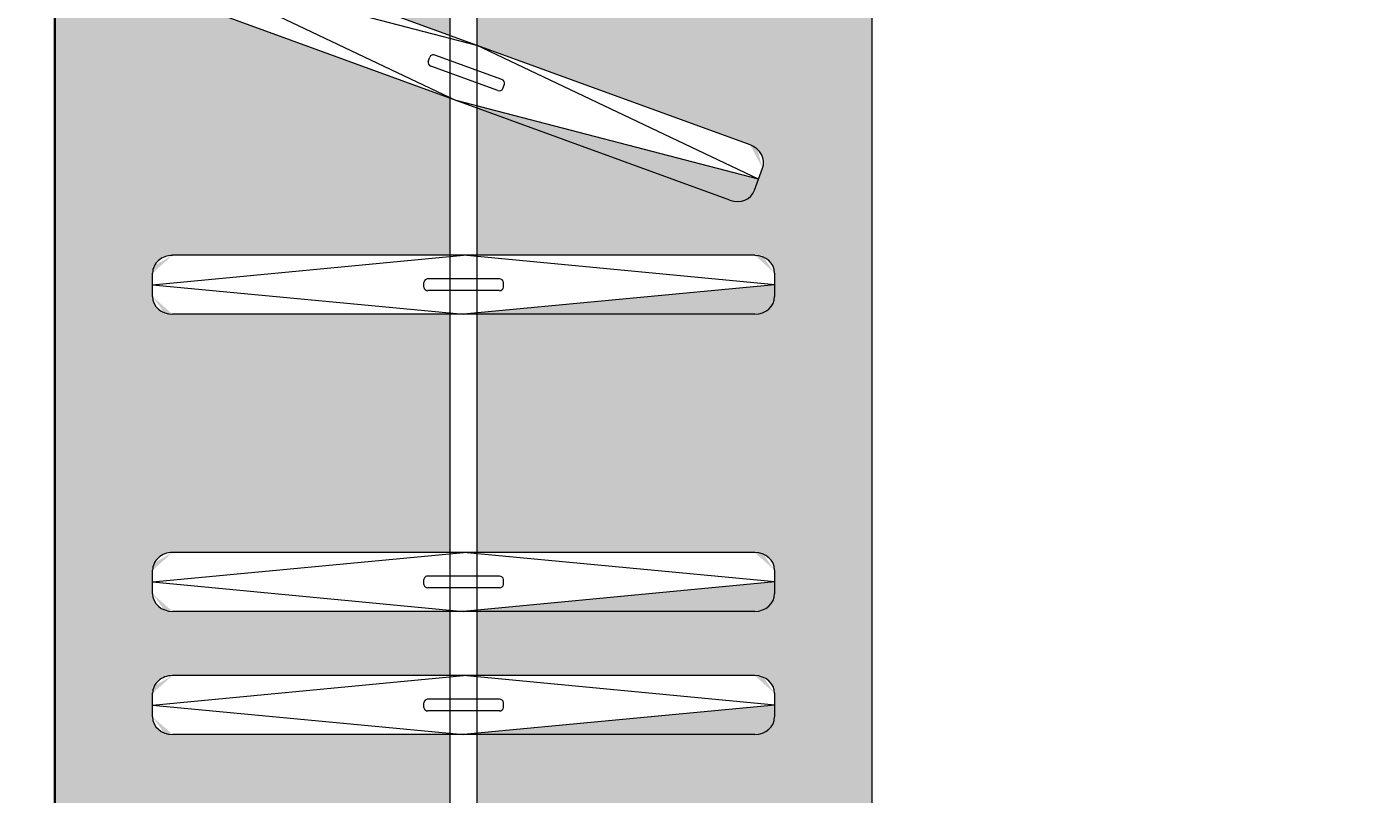
# Model space of a CAD drawing. Units: millimetres. Extents: x 27017497 to 27018854, y 7058029 to 7059154.
# Tile 66 of 91: x 27018319 to 27018355, y 7058154 to 7058174. Entities that reach past the tile are written whole.
import ezdxf

# ---------------------------------------------------------------- set-up
doc = ezdxf.new("R2010")
doc.units = ezdxf.units.MM
for name, color, linetype, lineweight in [('A-ANNO-DIMS', 2, 'Continuous', 18), ('A-FLOR-CASE', 8, 'Continuous', 20), ('A-FLOR-CASE-PATT', 44, 'Continuous', 13), ('A-WALL', 7, 'Continuous', 35)]:
    doc.layers.add(name, color=color, linetype=linetype, lineweight=lineweight)
doc.styles.get("Standard").update_dxf_attribs({"font": 'arial.ttf'})
doc.dimstyles.get("Standard").update_dxf_attribs({"dimtxt": 0.18, "dimasz": 0.18, "dimexe": 0.18, "dimexo": 0.0625, "dimgap": 0.09, "dimtad": 0, "dimtih": 1, "dimtoh": 1, "dimdec": 4, "dimzin": 0, "dimdsep": 46, "dimtxsty": 'Standard', "dimcen": 0.09, "dimadec": 0, "dimazin": 0, "dimtfac": 1, "dimtdec": 4, "dimtofl": 0, "dimtmove": 0, "dimatfit": 3, "dimfxl": 1, "dimtolj": 1, "dimtzin": 0, "dimarcsym": 0})

# ---------------------------------------------------------------- blocks, each defined once
blk = doc.blocks.new('WARDROBE-HANGING')
for p, q in [((0, 21.737), (65.212, 21.737)), ((39.589, 19.153), (38.806, 10.877)), ((39.902, 19.153), (39.276, 19.153)), ((39.589, 19.153), (40.372, 10.877)), ((47.493, 19.153), (46.71, 10.877)), ((47.806, 19.153), (47.18, 19.153)), ((47.493, 19.153), (48.276, 10.877)), ((50.766, 19.153), (49.984, 10.877)), ((51.079, 19.153), (50.453, 19.153)), ((50.766, 19.153), (51.549, 10.877)), ((36.783, 18.726), (33.217, 11.217)), ((36.783, 18.726), (34.688, 10.682)), ((37.077, 18.619), (36.488, 18.833)), ((38.806, 18.624), (38.806, 3.13)), ((40.372, 18.624), (40.372, 3.13)), ((46.71, 18.624), (46.71, 3.13)), ((48.276, 18.624), (48.276, 3.13)), ((49.984, 18.624), (49.984, 3.13)), ((51.549, 18.624), (51.549, 3.13)), ((35.867, 18.497), (30.567, 3.937)), ((37.337, 17.962), (32.038, 3.402)), ((34.13, 11.896), (33.48, 10.11)), ((34.372, 11.921), (34.255, 11.964)), ((39.432, 11.828), (39.432, 9.927)), ((39.652, 11.934), (39.526, 11.934)), ((39.745, 11.828), (39.745, 9.927)), ((47.336, 11.828), (47.336, 9.927)), ((47.556, 11.934), (47.43, 11.934)), ((47.649, 11.828), (47.649, 9.927)), ((50.61, 11.828), (50.61, 9.927)), ((50.829, 11.934), (50.704, 11.934)), ((50.923, 11.828), (50.923, 9.927)), ((34.425, 11.789), (33.774, 10.002)), ((0, 11.231), (65.212, 11.231)), ((31.122, 3.173), (33.217, 11.217)), ((39.589, 2.602), (38.806, 10.877)), ((39.589, 2.602), (40.372, 10.877)), ((47.493, 2.602), (46.71, 10.877)), ((47.493, 2.602), (48.276, 10.877)), ((50.766, 2.602), (49.984, 10.877)), ((50.766, 2.602), (51.549, 10.877)), ((0, 10.506), (65.212, 10.506)), ((31.122, 3.173), (34.688, 10.682)), ((33.65, 9.935), (33.532, 9.978)), ((39.652, 9.821), (39.526, 9.821)), ((47.556, 9.821), (47.43, 9.821)), ((50.829, 9.821), (50.704, 9.821)), ((39.902, 2.602), (39.276, 2.602)), ((47.806, 2.602), (47.18, 2.602)), ((51.079, 2.602), (50.453, 2.602)), ((0, 0), (65.212, 0))]:
    blk.add_line(p, q)
for centre, major_axis, start_param, end_param in [((39.276, 18.624), (0, 0.528), 0, 1.570796), ((39.902, 18.624), (0, 0.528), 4.712389, 6.283185), ((47.18, 18.624), (0, 0.528), 0, 1.570796), ((47.806, 18.624), (0, 0.528), 4.712389, 6.283185), ((50.453, 18.624), (0, 0.528), 0, 1.570796), ((51.079, 18.624), (0, 0.528), 4.712389, 6.283185), ((36.308, 18.336), (0.181, 0.496), 0, 1.570796), ((36.896, 18.122), (0.181, 0.496), -1.570796, 0), ((34.219, 11.864), (0.0361, 0.0993), 0, 1.570796), ((34.336, 11.821), (0.0361, 0.0993), 4.712389, 6.283185), ((39.526, 11.828), (0, 0.106), 0, 1.570796), ((39.652, 11.828), (0, 0.106), -1.570796, 0), ((47.43, 11.828), (0, 0.106), 0, 1.570796), ((47.556, 11.828), (0, 0.106), -1.570796, 0), ((50.704, 11.828), (0, 0.106), 0, 1.570796), ((50.829, 11.828), (0, 0.106), -1.570796, 0), ((33.568, 10.077), (0.0361, 0.0993), 1.570796, 3.141593), ((33.686, 10.035), (0.0361, 0.0993), 3.141593, 4.712389), ((39.526, 9.927), (0, 0.106), 1.570796, 3.141593), ((39.652, 9.927), (0, 0.106), 3.141593, 4.712389), ((47.43, 9.927), (0, 0.106), 1.570796, 3.141593), ((47.556, 9.927), (0, 0.106), 3.141593, 4.712389), ((50.704, 9.927), (0, 0.106), 1.570796, 3.141593), ((50.829, 9.927), (0, 0.106), 3.141593, 4.712389), ((39.276, 3.13), (0, 0.528), 1.570796, 3.141593), ((39.902, 3.13), (0, 0.528), 3.141593, 4.712389), ((47.18, 3.13), (0, 0.528), 1.570796, 3.141593), ((47.806, 3.13), (0, 0.528), 3.141593, 4.712389), ((50.453, 3.13), (0, 0.528), 1.570796, 3.141593), ((51.079, 3.13), (0, 0.528), 3.141593, 4.712389)]:
    blk.add_ellipse(centre, major_axis=major_axis, ratio=0.888892, start_param=start_param, end_param=end_param)
blk = doc.blocks.new('*D33')
at = {"layer": 'A-ANNO-DIMS', "color": 0, "lineweight": -2, "transparency": 16777216}
for p, q in [((27018319.543, 7058207.1), (27018309.644, 7058207.1)), ((27018309.824, 7058206.92), (27018309.824, 7058174.677)), ((27018309.824, 7058142.068), (27018309.824, 7058174.311)), ((27018319.543, 7058141.888), (27018309.644, 7058141.888))]:
    blk.add_line(p, q, dxfattribs=at)
at = {"layer": 'A-ANNO-DIMS', "color": 0, "transparency": 16777216}
for points in [[(27018309.794, 7058206.92), (27018309.854, 7058206.92), (27018309.824, 7058207.1)], [(27018309.794, 7058142.068), (27018309.854, 7058142.068), (27018309.824, 7058141.888)]]:
    blk.add_solid(points, dxfattribs=at)
at = {"layer": 'Defpoints', "color": 0, "transparency": 16777216}
for p in [(27018319.606, 7058207.1), (27018309.824, 7058141.888), (27018319.606, 7058141.888)]:
    blk.add_point(p, dxfattribs=at)
at = {"layer": 'A-ANNO-DIMS', "color": 0, "transparency": 16777216, "insert": (27018309.824, 7058174.494), "char_height": 0.18, "attachment_point": 5}
blk.add_mtext('\\A1;WARDROBE 65 TYP.', dxfattribs=at)
blk = doc.blocks.new('*D47')
at = {"layer": 'A-ANNO-DIMS', "color": 0, "lineweight": -2, "transparency": 16777216}
for p, q in [((27017561.166, 7058294.35), (27017561.166, 7058028.6)), ((27018790.606, 7058294.35), (27018790.606, 7058028.6)), ((27017561.346, 7058028.78), (27018175.431, 7058028.78)), ((27018790.426, 7058028.78), (27018176.341, 7058028.78))]:
    blk.add_line(p, q, dxfattribs=at)
at = {"layer": 'A-ANNO-DIMS', "color": 0, "transparency": 16777216}
for points in [[(27017561.346, 7058028.81), (27017561.346, 7058028.75), (27017561.166, 7058028.78)], [(27018790.426, 7058028.81), (27018790.426, 7058028.75), (27018790.606, 7058028.78)]]:
    blk.add_solid(points, dxfattribs=at)
at = {"layer": 'Defpoints', "color": 0, "transparency": 16777216}
for p in [(27017561.166, 7058294.412), (27018790.606, 7058294.412), (27018790.606, 7058028.78)]:
    blk.add_point(p, dxfattribs=at)
at = {"layer": 'A-ANNO-DIMS', "color": 0, "transparency": 16777216, "insert": (27018175.886, 7058028.78), "char_height": 0.18, "attachment_point": 5}
blk.add_mtext('\\A1;1229.4', dxfattribs=at)
blk = doc.blocks.new('*D48')
at = {"layer": 'A-ANNO-DIMS', "color": 0, "lineweight": -2, "transparency": 16777216}
for p, q in [((27018463.498, 7058622.912), (27017497.536, 7058622.912)), ((27017497.716, 7058622.732), (27017497.716, 7058357.753)), ((27017497.716, 7058092.41), (27017497.716, 7058357.389)), ((27018555.129, 7058092.23), (27017497.536, 7058092.23))]:
    blk.add_line(p, q, dxfattribs=at)
at = {"layer": 'A-ANNO-DIMS', "color": 0, "transparency": 16777216}
for points in [[(27017497.686, 7058622.732), (27017497.746, 7058622.732), (27017497.716, 7058622.912)], [(27017497.686, 7058092.41), (27017497.746, 7058092.41), (27017497.716, 7058092.23)]]:
    blk.add_solid(points, dxfattribs=at)
at = {"layer": 'Defpoints', "color": 0, "transparency": 16777216}
for p in [(27018463.561, 7058622.912), (27017497.716, 7058092.23), (27018555.192, 7058092.23)]:
    blk.add_point(p, dxfattribs=at)
at = {"layer": 'A-ANNO-DIMS', "color": 0, "transparency": 16777216, "insert": (27017497.716, 7058357.571), "char_height": 0.18, "attachment_point": 5}
blk.add_mtext('\\A1;530.7', dxfattribs=at)

msp = doc.modelspace()

# ---------------------------------------------------------------- hatches: boundary and pattern name
at = {"layer": 'A-FLOR-CASE-PATT'}
h = msp.add_hatch(color=256, dxfattribs=at)
h.dxf.hatch_style = 1
edge = h.paths.add_edge_path()
edge.add_line((27018341.343, 7058207.055), (27018330.837, 7058207.055))
edge.add_line((27018330.837, 7058207.055), (27018330.837, 7058203.02))
edge.add_line((27018330.837, 7058203.02), (27018338.424, 7058203.02))
edge.add_ellipse((27018338.23, 7058202.551), major_axis=(0.528, 0), ratio=0.888892, start_angle=0, end_angle=90, ccw=False)
edge.add_line((27018338.758, 7058202.551), (27018338.758, 7058202.238))
edge.add_line((27018338.758, 7058202.238), (27018330.837, 7058201.488))
edge.add_line((27018330.837, 7058201.488), (27018330.837, 7058199.747))
edge.add_line((27018330.837, 7058199.747), (27018338.424, 7058199.747))
edge.add_ellipse((27018338.23, 7058199.277), major_axis=(0.528, 0), ratio=0.888892, start_angle=0, end_angle=90, ccw=False)
edge.add_line((27018338.758, 7058199.277), (27018338.758, 7058198.964))
edge.add_line((27018338.758, 7058198.964), (27018330.837, 7058198.215))
edge.add_line((27018330.837, 7058198.215), (27018330.837, 7058193.415))
edge.add_line((27018330.837, 7058193.415), (27018338.284, 7058190.704))
edge.add_ellipse((27018337.942, 7058190.329), major_axis=(0.496, -0.181), ratio=0.888892, start_angle=0, end_angle=90, ccw=False)
edge.add_line((27018338.439, 7058190.148), (27018338.331, 7058189.854))
edge.add_line((27018338.331, 7058189.854), (27018330.837, 7058191.806))
edge.add_line((27018330.837, 7058191.806), (27018330.837, 7058188.22))
edge.add_line((27018330.837, 7058188.22), (27018338.424, 7058188.22))
edge.add_ellipse((27018338.23, 7058187.75), major_axis=(0.528, 0), ratio=0.888892, start_angle=0, end_angle=90, ccw=False)
edge.add_line((27018338.758, 7058187.75), (27018338.758, 7058187.437))
edge.add_line((27018338.758, 7058187.437), (27018330.837, 7058186.688))
edge.add_line((27018330.837, 7058186.688), (27018330.837, 7058181.982))
edge.add_line((27018330.837, 7058181.982), (27018338.424, 7058181.982))
edge.add_ellipse((27018338.23, 7058181.513), major_axis=(0.528, 0), ratio=0.888892, start_angle=0, end_angle=90, ccw=False)
edge.add_line((27018338.758, 7058181.513), (27018338.758, 7058181.199))
edge.add_line((27018338.758, 7058181.199), (27018330.837, 7058180.45))
edge.add_line((27018330.837, 7058180.45), (27018330.837, 7058178.709))
edge.add_line((27018330.837, 7058178.709), (27018338.424, 7058178.709))
edge.add_ellipse((27018338.23, 7058178.239), major_axis=(0.528, 0), ratio=0.888892, start_angle=0, end_angle=90, ccw=False)
edge.add_line((27018338.758, 7058178.239), (27018338.758, 7058177.926))
edge.add_line((27018338.758, 7058177.926), (27018330.837, 7058177.177))
edge.add_line((27018330.837, 7058177.177), (27018330.837, 7058173.878))
edge.add_line((27018330.837, 7058173.878), (27018338.284, 7058171.167))
edge.add_ellipse((27018337.942, 7058170.792), major_axis=(0.496, -0.181), ratio=0.888892, start_angle=0, end_angle=90, ccw=False)
edge.add_line((27018338.439, 7058170.611), (27018338.331, 7058170.317))
edge.add_line((27018338.331, 7058170.317), (27018330.837, 7058172.269))
edge.add_line((27018330.837, 7058172.269), (27018330.837, 7058168.293))
edge.add_line((27018330.837, 7058168.293), (27018338.424, 7058168.293))
edge.add_ellipse((27018338.23, 7058167.824), major_axis=(0.528, 0), ratio=0.888892, start_angle=0, end_angle=90, ccw=False)
edge.add_line((27018338.758, 7058167.824), (27018338.758, 7058167.511))
edge.add_line((27018338.758, 7058167.511), (27018330.837, 7058166.762))
edge.add_line((27018330.837, 7058166.762), (27018330.837, 7058160.389))
edge.add_line((27018330.837, 7058160.389), (27018338.424, 7058160.389))
edge.add_ellipse((27018338.23, 7058159.92), major_axis=(0.528, 0), ratio=0.888892, start_angle=0, end_angle=90, ccw=False)
edge.add_line((27018338.758, 7058159.92), (27018338.758, 7058159.607))
edge.add_line((27018338.758, 7058159.607), (27018330.837, 7058158.858))
edge.add_line((27018330.837, 7058158.858), (27018330.837, 7058157.116))
edge.add_line((27018330.837, 7058157.116), (27018338.424, 7058157.116))
edge.add_ellipse((27018338.23, 7058156.647), major_axis=(0.528, 0), ratio=0.888892, start_angle=0, end_angle=90, ccw=False)
edge.add_line((27018338.758, 7058156.647), (27018338.758, 7058156.334))
edge.add_line((27018338.758, 7058156.334), (27018330.837, 7058155.585))
edge.add_line((27018330.837, 7058155.585), (27018330.837, 7058150.784))
edge.add_line((27018330.837, 7058150.784), (27018338.284, 7058148.073))
edge.add_ellipse((27018337.942, 7058147.698), major_axis=(0.496, -0.181), ratio=0.888892, start_angle=0, end_angle=90, ccw=False)
edge.add_line((27018338.439, 7058147.517), (27018338.331, 7058147.223))
edge.add_line((27018338.331, 7058147.223), (27018330.837, 7058149.175))
edge.add_line((27018330.837, 7058149.175), (27018330.837, 7058145.589))
edge.add_line((27018330.837, 7058145.589), (27018338.424, 7058145.589))
edge.add_ellipse((27018338.23, 7058145.119), major_axis=(0.528, 0), ratio=0.888892, start_angle=0, end_angle=90, ccw=False)
edge.add_line((27018338.758, 7058145.119), (27018338.758, 7058144.806))
edge.add_line((27018338.758, 7058144.806), (27018330.837, 7058144.057))
edge.add_line((27018330.837, 7058144.057), (27018330.837, 7058141.912))
edge.add_line((27018330.837, 7058141.912), (27018341.343, 7058141.912))
edge.add_line((27018341.343, 7058141.912), (27018341.343, 7058207.055))
edge = h.paths.add_edge_path()
edge.add_line((27018330.112, 7058207.055), (27018319.606, 7058207.055))
edge.add_line((27018319.606, 7058207.055), (27018319.606, 7058141.912))
edge.add_line((27018319.606, 7058141.912), (27018330.112, 7058141.912))
edge.add_line((27018330.112, 7058141.912), (27018330.112, 7058144.024))
edge.add_line((27018330.112, 7058144.024), (27018322.543, 7058144.024))
edge.add_ellipse((27018322.736, 7058144.493), major_axis=(0.528, 0), ratio=0.888892, start_angle=180, end_angle=270, ccw=False)
edge.add_line((27018322.208, 7058144.493), (27018322.208, 7058145.291))
edge.add_ellipse((27018322.736, 7058145.119), major_axis=(0.528, 0), ratio=0.888892, start_angle=90, end_angle=180, ccw=False)
edge.add_line((27018322.736, 7058145.589), (27018330.112, 7058145.589))
edge.add_line((27018330.112, 7058145.589), (27018330.112, 7058149.382))
edge.add_line((27018330.112, 7058149.382), (27018322.826, 7058152.034))
edge.add_ellipse((27018323.168, 7058152.409), major_axis=(0.496, -0.181), ratio=0.888892, start_angle=180, end_angle=270, ccw=False)
edge.add_line((27018322.672, 7058152.59), (27018322.945, 7058153.34))
edge.add_ellipse((27018323.382, 7058152.997), major_axis=(0.496, -0.181), ratio=0.888892, start_angle=90, end_angle=180, ccw=False)
edge.add_line((27018323.543, 7058153.439), (27018330.112, 7058151.048))
edge.add_line((27018330.112, 7058151.048), (27018330.112, 7058155.551))
edge.add_line((27018330.112, 7058155.551), (27018322.543, 7058155.551))
edge.add_ellipse((27018322.736, 7058156.021), major_axis=(0.528, 0), ratio=0.888892, start_angle=180, end_angle=270, ccw=False)
edge.add_line((27018322.208, 7058156.021), (27018322.208, 7058156.819))
edge.add_ellipse((27018322.736, 7058156.647), major_axis=(0.528, 0), ratio=0.888892, start_angle=90, end_angle=180, ccw=False)
edge.add_line((27018322.736, 7058157.116), (27018330.112, 7058157.116))
edge.add_line((27018330.112, 7058157.116), (27018330.112, 7058158.824))
edge.add_line((27018330.112, 7058158.824), (27018322.543, 7058158.824))
edge.add_ellipse((27018322.736, 7058159.294), major_axis=(0.528, 0), ratio=0.888892, start_angle=180, end_angle=270, ccw=False)
edge.add_line((27018322.208, 7058159.294), (27018322.208, 7058160.092))
edge.add_ellipse((27018322.736, 7058159.92), major_axis=(0.528, 0), ratio=0.888892, start_angle=90, end_angle=180, ccw=False)
edge.add_line((27018322.736, 7058160.389), (27018330.112, 7058160.389))
edge.add_line((27018330.112, 7058160.389), (27018330.112, 7058166.728))
edge.add_line((27018330.112, 7058166.728), (27018322.543, 7058166.728))
edge.add_ellipse((27018322.736, 7058167.198), major_axis=(0.528, 0), ratio=0.888892, start_angle=180, end_angle=270, ccw=False)
edge.add_line((27018322.208, 7058167.198), (27018322.208, 7058167.996))
edge.add_ellipse((27018322.736, 7058167.824), major_axis=(0.528, 0), ratio=0.888892, start_angle=90, end_angle=180, ccw=False)
edge.add_line((27018322.736, 7058168.293), (27018330.112, 7058168.293))
edge.add_line((27018330.112, 7058168.293), (27018330.112, 7058172.476))
edge.add_line((27018330.112, 7058172.476), (27018322.826, 7058175.128))
edge.add_ellipse((27018323.168, 7058175.503), major_axis=(0.496, -0.181), ratio=0.888892, start_angle=180, end_angle=270, ccw=False)
edge.add_line((27018322.672, 7058175.684), (27018322.945, 7058176.433))
edge.add_ellipse((27018323.382, 7058176.091), major_axis=(0.496, -0.181), ratio=0.888892, start_angle=90, end_angle=180, ccw=False)
edge.add_line((27018323.543, 7058176.533), (27018330.112, 7058174.142))
edge.add_line((27018330.112, 7058174.142), (27018330.112, 7058177.144))
edge.add_line((27018330.112, 7058177.144), (27018322.543, 7058177.144))
edge.add_ellipse((27018322.736, 7058177.613), major_axis=(0.528, 0), ratio=0.888892, start_angle=180, end_angle=270, ccw=False)
edge.add_line((27018322.208, 7058177.613), (27018322.208, 7058178.411))
edge.add_ellipse((27018322.736, 7058178.239), major_axis=(0.528, 0), ratio=0.888892, start_angle=90, end_angle=180, ccw=False)
edge.add_line((27018322.736, 7058178.709), (27018330.112, 7058178.709))
edge.add_line((27018330.112, 7058178.709), (27018330.112, 7058180.417))
edge.add_line((27018330.112, 7058180.417), (27018322.543, 7058180.417))
edge.add_ellipse((27018322.736, 7058180.886), major_axis=(0.528, 0), ratio=0.888892, start_angle=180, end_angle=270, ccw=False)
edge.add_line((27018322.208, 7058180.886), (27018322.208, 7058181.684))
edge.add_ellipse((27018322.736, 7058181.513), major_axis=(0.528, 0), ratio=0.888892, start_angle=90, end_angle=180, ccw=False)
edge.add_line((27018322.736, 7058181.982), (27018330.112, 7058181.982))
edge.add_line((27018330.112, 7058181.982), (27018330.112, 7058186.655))
edge.add_line((27018330.112, 7058186.655), (27018322.543, 7058186.655))
edge.add_ellipse((27018322.736, 7058187.124), major_axis=(0.528, 0), ratio=0.888892, start_angle=180, end_angle=270, ccw=False)
edge.add_line((27018322.208, 7058187.124), (27018322.208, 7058187.922))
edge.add_ellipse((27018322.736, 7058187.75), major_axis=(0.528, 0), ratio=0.888892, start_angle=90, end_angle=180, ccw=False)
edge.add_line((27018322.736, 7058188.22), (27018330.112, 7058188.22))
edge.add_line((27018330.112, 7058188.22), (27018330.112, 7058192.013))
edge.add_line((27018330.112, 7058192.013), (27018322.826, 7058194.665))
edge.add_ellipse((27018323.168, 7058195.04), major_axis=(0.496, -0.181), ratio=0.888892, start_angle=180, end_angle=270, ccw=False)
edge.add_line((27018322.672, 7058195.22), (27018322.945, 7058195.97))
edge.add_ellipse((27018323.382, 7058195.628), major_axis=(0.496, -0.181), ratio=0.888892, start_angle=90, end_angle=180, ccw=False)
edge.add_line((27018323.543, 7058196.069), (27018330.112, 7058193.678))
edge.add_line((27018330.112, 7058193.678), (27018330.112, 7058198.182))
edge.add_line((27018330.112, 7058198.182), (27018322.543, 7058198.182))
edge.add_ellipse((27018322.736, 7058198.651), major_axis=(0.528, 0), ratio=0.888892, start_angle=180, end_angle=270, ccw=False)
edge.add_line((27018322.208, 7058198.651), (27018322.208, 7058199.449))
edge.add_ellipse((27018322.736, 7058199.277), major_axis=(0.528, 0), ratio=0.888892, start_angle=90, end_angle=180, ccw=False)
edge.add_line((27018322.736, 7058199.747), (27018330.112, 7058199.747))
edge.add_line((27018330.112, 7058199.747), (27018330.112, 7058201.455))
edge.add_line((27018330.112, 7058201.455), (27018322.543, 7058201.455))
edge.add_ellipse((27018322.736, 7058201.924), major_axis=(0.528, 0), ratio=0.888892, start_angle=180, end_angle=270, ccw=False)
edge.add_line((27018322.208, 7058201.924), (27018322.208, 7058202.722))
edge.add_ellipse((27018322.736, 7058202.551), major_axis=(0.528, 0), ratio=0.888892, start_angle=90, end_angle=180, ccw=False)
edge.add_line((27018322.736, 7058203.02), (27018330.112, 7058203.02))
edge.add_line((27018330.112, 7058203.02), (27018330.112, 7058207.055))
h.paths.add_polyline_path([(27018341.31, 7058294.412), (27018319.606, 7058294.412), (27018319.606, 7058207.1), (27018341.31, 7058207.1)])
h.paths.add_polyline_path([(27018354.358, 7058255.592), (27018354.358, 7058256.057, -0.414214), (27018354.869, 7058256.569), (27018346.477, 7058256.569, -0.414214), (27018345.197, 7058257.848), (27018345.197, 7058259.128, -0.414214), (27018346.477, 7058260.407), (27018343.868, 7058260.407, 0.290979), (27018341.551, 7058258.934), (27018341.551, 7058242.534, 0.290979), (27018343.868, 7058241.06), (27018346.477, 7058241.06, -0.414214), (27018345.197, 7058242.34), (27018345.197, 7058243.619, -0.414214), (27018346.477, 7058244.899), (27018353.078, 7058244.899, 0.414214), (27018354.358, 7058246.178)])
h.paths.add_polyline_path([(27018356.917, 7058260.407), (27018346.477, 7058260.407, 0.414214), (27018345.197, 7058259.128), (27018345.197, 7058257.848, 0.414214), (27018346.477, 7058256.569), (27018355.637, 7058256.569), (27018355.637, 7058244.899), (27018346.477, 7058244.899, 0.414214), (27018345.197, 7058243.619), (27018345.197, 7058242.34, 0.414214), (27018346.477, 7058241.06), (27018356.917, 7058241.06, 0.414214), (27018359.476, 7058243.619), (27018359.476, 7058257.848, 0.414214)])
h.paths.add_polyline_path([(27018355.637, 7058252.362), (27018355.637, 7058256.057, 0.490314), (27018354.997, 7058256.553, 0.490314), (27018354.358, 7058256.057), (27018354.358, 7058255.592), (27018354.358, 7058245.411, 0.490314), (27018354.997, 7058244.915, 0.490314), (27018355.637, 7058245.411)], flags=17)

# ---------------------------------------------------------------- linework, layer by layer
at = {"layer": 'A-WALL'}
msp.add_line((27018319.606, 7058386.803), (27018319.606, 7058141.912), dxfattribs=at)

# ---------------------------------------------------------------- block references
at = {"layer": 'A-FLOR-CASE', "rotation": 270}
msp.add_blockref('WARDROBE-HANGING', (27018319.606, 7058207.1), dxfattribs=at)

# ---------------------------------------------------------------- dimensions: what is measured, and where the dimension line sits
at = {"layer": 'A-ANNO-DIMS'}
dim = msp.add_linear_dim(base=(27017497.716, 7058092.23), p1=(27018463.561, 7058622.912), p2=(27018555.192, 7058092.23), angle=90, dimstyle='Standard', override={"dimdec": 1, "dimlfac": 1, "dimrnd": 0, "dimzin": 0, "dimdsep": 46, "dimlunit": 2}, dxfattribs=at)
dim.commit()
dim.dimension.update_dxf_attribs({"geometry": '*D48', "text_midpoint": (27017497.716, 7058357.571)})
dim = msp.add_linear_dim(base=(27018790.606, 7058028.78), p1=(27017561.166, 7058294.412), p2=(27018790.606, 7058294.412), dimstyle='Standard', override={"dimdec": 1, "dimlfac": 1, "dimrnd": 0, "dimzin": 0, "dimdsep": 46, "dimlunit": 2}, dxfattribs=at)
dim.commit()
dim.dimension.update_dxf_attribs({"geometry": '*D47', "text_midpoint": (27018175.886, 7058028.78)})
dim = msp.add_linear_dim(base=(27018309.824, 7058141.888), p1=(27018319.606, 7058207.1), p2=(27018319.606, 7058141.888), angle=270, text='WARDROBE <> TYP.', dimstyle='Standard', override={"dimdec": 0, "dimlfac": 1, "dimrnd": 0, "dimzin": 0, "dimdsep": 46, "dimlunit": 2}, dxfattribs=at)
dim.commit()
dim.dimension.update_dxf_attribs({"geometry": '*D33', "text_midpoint": (27018309.824, 7058174.494)})

doc.saveas('drawing.dxf')
